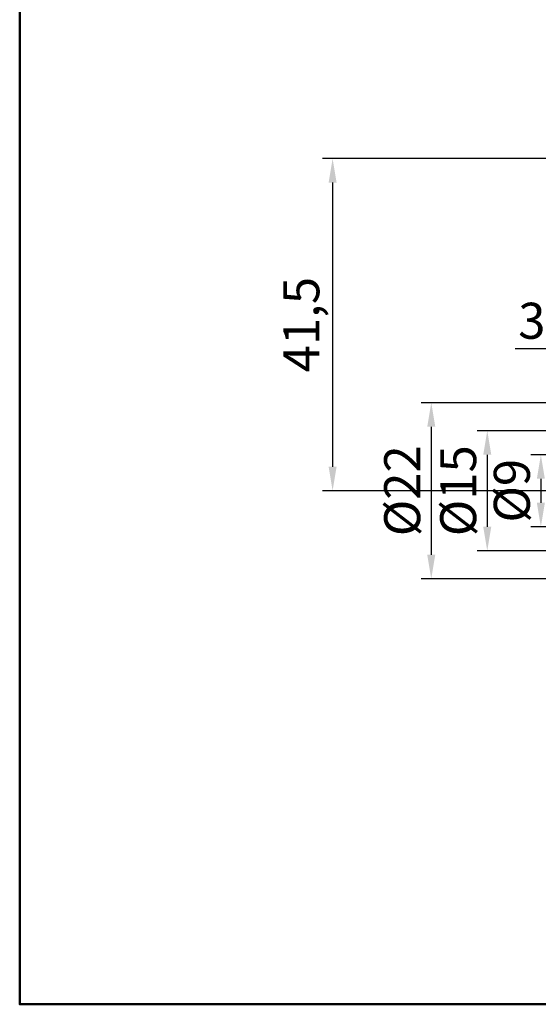
# Model space of a CAD drawing. Units: millimetres. Extents: x 418 to 773, y -46 to 294.
# Tile 1 of 7: x 418 to 483, y -46 to 77. Entities that reach past the tile are written whole.
import ezdxf

# ---------------------------------------------------------------- set-up
doc = ezdxf.new("R2010")
doc.units = ezdxf.units.MM
doc.header["$LTSCALE"] = 0.2
doc.layers.add('M-DIMS', color=2, linetype='Continuous', lineweight=25)
doc.layers.add('M-TTLB', color=7, linetype='Continuous', lineweight=50)
doc.styles.get("Standard").update_dxf_attribs({"font": 'arial.ttf'})
doc.dimstyles.new('ISO-25', dxfattribs={"dimtxt": 4.5, "dimasz": 3, "dimexe": 1.25, "dimexo": 0.625, "dimtad": 1, "dimdec": 1, "dimtxsty": 'Standard', "dimcen": 2.5, "dimadec": 0, "dimazin": 0, "dimtfac": 1, "dimtdec": 1, "dimtmove": 0, "dimatfit": 3, "dimfxl": 1, "dimarcsym": 0})

# ---------------------------------------------------------------- blocks, each defined once
blk = doc.blocks.new('*D71')
at = {"layer": 'Defpoints', "color": 0, "ltscale": 0.2, "transparency": 16777216}
for p in [(490.05, 22.18), (483.08, 13.18), (490.05, 13.18)]:
    blk.add_point(p, dxfattribs=at)
at = {"layer": 'M-DIMS', "color": 0, "lineweight": -2, "ltscale": 0.2, "transparency": 16777216}
for p, q in [((489.42, 22.18), (481.83, 22.18)), ((483.08, 19.18), (483.08, 16.18)), ((489.42, 13.18), (481.83, 13.18))]:
    blk.add_line(p, q, dxfattribs=at)
at = {"layer": 'M-DIMS', "color": 0, "ltscale": 0.2, "transparency": 16777216}
for points in [[(482.58, 19.18), (483.58, 19.18), (483.08, 22.18)], [(482.58, 16.18), (483.58, 16.18), (483.08, 13.18)]]:
    blk.add_solid(points, dxfattribs=at)
at = {"layer": 'M-DIMS', "color": 0, "ltscale": 0.2, "transparency": 16777216, "insert": (480.03, 17.68), "char_height": 4.5, "attachment_point": 5, "rotation": 90}
blk.add_mtext('%%C9', dxfattribs=at)
blk = doc.blocks.new('*D72')
at = {"layer": 'Defpoints', "color": 0, "ltscale": 0.2, "transparency": 16777216}
for p in [(490.05, 25.18), (476.38, 10.18), (490.05, 10.18)]:
    blk.add_point(p, dxfattribs=at)
at = {"layer": 'M-DIMS', "color": 0, "lineweight": -2, "ltscale": 0.2, "transparency": 16777216}
for p, q in [((489.42, 25.18), (475.13, 25.18)), ((476.38, 22.18), (476.38, 13.18)), ((489.42, 10.18), (475.13, 10.18))]:
    blk.add_line(p, q, dxfattribs=at)
at = {"layer": 'M-DIMS', "color": 0, "ltscale": 0.2, "transparency": 16777216}
for points in [[(475.88, 22.18), (476.88, 22.18), (476.38, 25.18)], [(475.88, 13.18), (476.88, 13.18), (476.38, 10.18)]]:
    blk.add_solid(points, dxfattribs=at)
at = {"layer": 'M-DIMS', "color": 0, "ltscale": 0.2, "transparency": 16777216, "insert": (473.33, 17.68), "char_height": 4.5, "attachment_point": 5, "rotation": 90}
blk.add_mtext('%%C15', dxfattribs=at)
blk = doc.blocks.new('*D73')
at = {"layer": 'Defpoints', "color": 0, "ltscale": 0.2, "transparency": 16777216}
for p in [(490.05, 28.68), (469.38, 6.68), (490.05, 6.68)]:
    blk.add_point(p, dxfattribs=at)
at = {"layer": 'M-DIMS', "color": 0, "lineweight": -2, "ltscale": 0.2, "transparency": 16777216}
for p, q in [((489.42, 28.68), (468.13, 28.68)), ((469.38, 25.68), (469.38, 9.68)), ((489.42, 6.68), (468.13, 6.68))]:
    blk.add_line(p, q, dxfattribs=at)
at = {"layer": 'M-DIMS', "color": 0, "ltscale": 0.2, "transparency": 16777216}
for points in [[(468.88, 25.68), (469.88, 25.68), (469.38, 28.68)], [(468.88, 9.68), (469.88, 9.68), (469.38, 6.68)]]:
    blk.add_solid(points, dxfattribs=at)
at = {"layer": 'M-DIMS', "color": 0, "ltscale": 0.2, "transparency": 16777216, "insert": (466.33, 17.68), "char_height": 4.5, "attachment_point": 5, "rotation": 90}
blk.add_mtext('%%C22', dxfattribs=at)
blk = doc.blocks.new('*D78')
at = {"layer": 'Defpoints', "color": 0, "ltscale": 0.2, "transparency": 16777216}
for p in [(493.05, 35.4), (490.05, 28.68), (493.05, 28.68)]:
    blk.add_point(p, dxfattribs=at)
at = {"layer": 'M-DIMS', "color": 0, "lineweight": -2, "ltscale": 0.2, "transparency": 16777216}
for p, q in [((490.05, 29.31), (490.05, 36.65)), ((493.05, 29.31), (493.05, 36.65)), ((487.05, 35.4), (479.85, 35.4)), ((493.05, 35.4), (490.05, 35.4)), ((496.05, 35.4), (499.05, 35.4))]:
    blk.add_line(p, q, dxfattribs=at)
at = {"layer": 'M-DIMS', "color": 0, "ltscale": 0.2, "transparency": 16777216}
for points in [[(487.05, 35.9), (487.05, 34.9), (490.05, 35.4)], [(496.05, 35.9), (496.05, 34.9), (493.05, 35.4)]]:
    blk.add_solid(points, dxfattribs=at)
at = {"layer": 'M-DIMS', "color": 0, "ltscale": 0.2, "transparency": 16777216, "insert": (481.95, 38.33), "char_height": 4.5, "attachment_point": 5}
blk.add_mtext('3', dxfattribs=at)
blk = doc.blocks.new('*D86')
at = {"layer": 'Defpoints', "color": 0, "ltscale": 0.2, "transparency": 16777216}
for p in [(525.05, 59.18), (457.05, 17.68), (525.05, 17.68)]:
    blk.add_point(p, dxfattribs=at)
at = {"layer": 'M-DIMS', "color": 0, "lineweight": -2, "ltscale": 0.2, "transparency": 16777216}
for p, q in [((524.42, 59.18), (455.8, 59.18)), ((457.05, 56.18), (457.05, 20.68)), ((524.42, 17.68), (455.8, 17.68))]:
    blk.add_line(p, q, dxfattribs=at)
at = {"layer": 'M-DIMS', "color": 0, "ltscale": 0.2, "transparency": 16777216}
for points in [[(456.55, 56.18), (457.55, 56.18), (457.05, 59.18)], [(456.55, 20.68), (457.55, 20.68), (457.05, 17.68)]]:
    blk.add_solid(points, dxfattribs=at)
at = {"layer": 'M-DIMS', "color": 0, "ltscale": 0.2, "transparency": 16777216, "insert": (453.72, 38.43), "char_height": 4.5, "attachment_point": 5, "rotation": 90}
blk.add_mtext('41,5', dxfattribs=at)

msp = doc.modelspace()

# ---------------------------------------------------------------- linework, layer by layer
at = {"layer": 'M-TTLB', "ltscale": 0.2}
msp.add_lwpolyline([(417.9371, 294.4119), (773.2687, 294.4119), (773.2687, -46.4726), (417.9371, -46.4726)], close=True, dxfattribs=at)

# ---------------------------------------------------------------- dimensions: what is measured, and where the dimension line sits
at = {"layer": 'M-DIMS', "ltscale": 0.2}
dim = msp.add_linear_dim(base=(457.0454, 17.6849), p1=(525.0464, 59.1849), p2=(525.0464, 17.6849), angle=90, dimstyle='ISO-25', override={"dimclrd": 0, "dimclre": 0, "dimclrt": 0}, dxfattribs=at)
dim.commit()
dim.dimension.update_dxf_attribs({"geometry": '*D86', "text_midpoint": (453.7161, 38.4349)})
dim = msp.add_linear_dim(base=(493.0464, 35.4018), p1=(490.0464, 28.6849), p2=(493.0464, 28.6849), dimstyle='ISO-25', override={"dimclrd": 0, "dimclre": 0, "dimclrt": 0}, dxfattribs=at)
dim.commit()
dim.dimension.update_dxf_attribs({"geometry": '*D78', "text_midpoint": (481.948, 35.4018), "dimtype": 160})
for base, p1, p2, picture, middle in [((469.3802, 6.6849), (490.0464, 28.6849), (490.0464, 6.6849), '*D73', (466.3318, 17.6849)), ((476.377, 10.1849), (490.0464, 25.1849), (490.0464, 10.1849), '*D72', (473.3286, 17.6849))]:
    dim = msp.add_linear_dim(base=base, p1=p1, p2=p2, angle=90, text='%%C<>', dimstyle='ISO-25', override={"dimclrd": 0, "dimclre": 0, "dimclrt": 0}, dxfattribs=at)
    dim.commit()
    dim.dimension.update_dxf_attribs({"geometry": picture, "text_midpoint": middle})
dim = msp.add_linear_dim(base=(483.0819, 13.1849), p1=(490.0464, 22.1849), p2=(490.0464, 13.1849), angle=90, text='%%C<>', dimstyle='ISO-25', override={"dimclrd": 0, "dimclre": 0, "dimclrt": 0}, dxfattribs=at)
dim.commit()
dim.dimension.update_dxf_attribs({"geometry": '*D71', "text_midpoint": (483.0819, 17.6849), "dimtype": 160})

doc.saveas('drawing.dxf')
